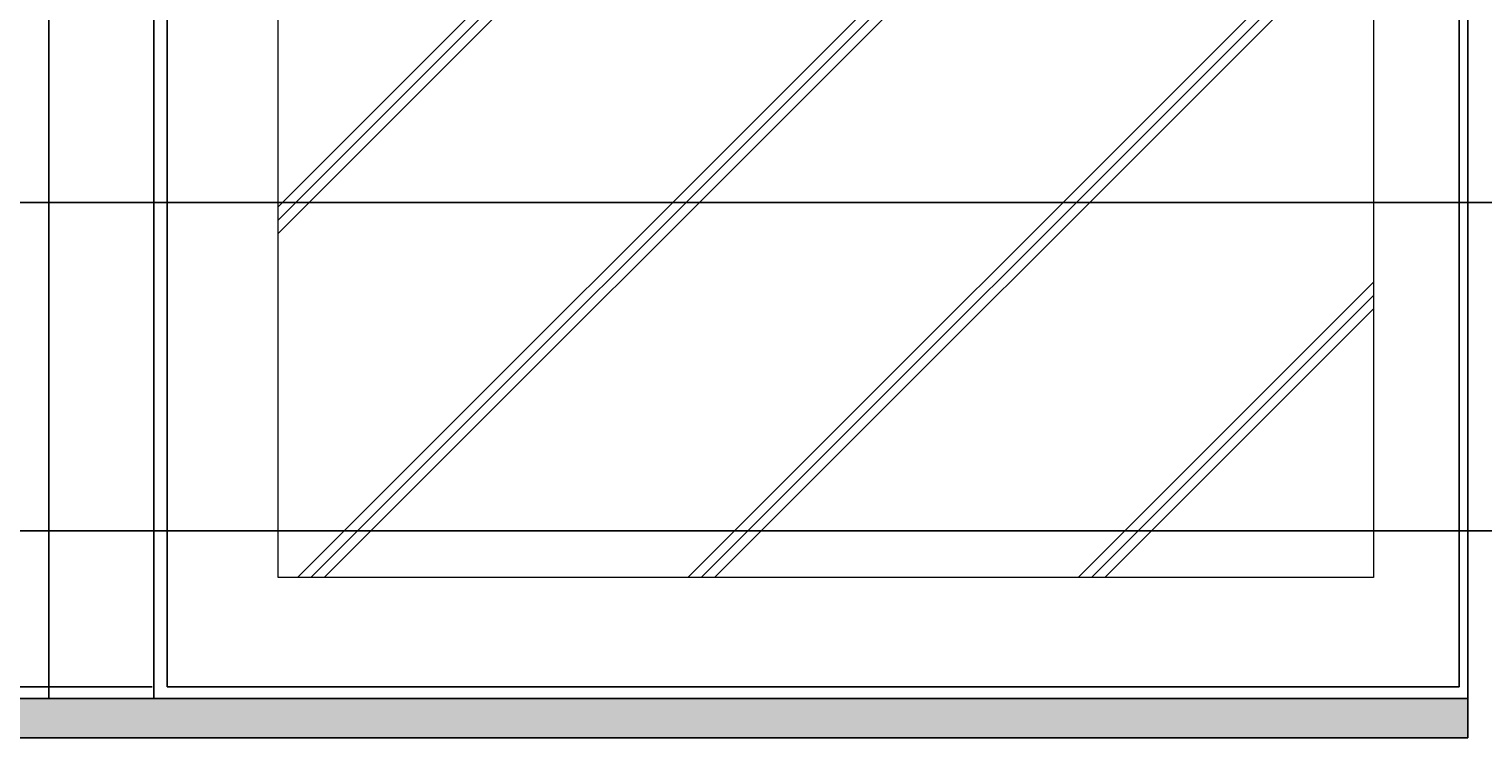
# Model space of a CAD drawing. Units: millimetres. Extents: x 2332 to 5836, y -853 to 2199.
# Tile 3 of 16: x 3088 to 3641, y 753 to 1023. Entities that reach past the tile are written whole.
import ezdxf

# ---------------------------------------------------------------- set-up
doc = ezdxf.new("R2010")
doc.units = ezdxf.units.MM
doc.layers.get('0').update_dxf_attribs({"color": 8})
for name, color, linetype, lineweight in [('A-ANNO-DIMS', 2, 'Continuous', 18), ('A-CSWK-GLAZ', 7, 'Continuous', 18), ('A-CSWK-PATT', 40, 'Continuous', 13), ('A-GLAZ-PATT', 4, 'Continuous', 13), ('SHELF', 40, 'Continuous', 25)]:
    doc.layers.add(name, color=color, linetype=linetype, lineweight=lineweight)
doc.styles.get("Standard").update_dxf_attribs({"font": 'arial.ttf'})
doc.dimstyles.new('ISO-25', dxfattribs={"dimtxt": 2.5, "dimasz": 2.5, "dimexe": 1.25, "dimexo": 0.625, "dimtad": 1, "dimtxsty": 'Standard', "dimcen": 2.5, "dimadec": 0, "dimazin": 0, "dimtfac": 1, "dimtmove": 0, "dimatfit": 3, "dimfxl": 1, "dimarcsym": 0})

# ---------------------------------------------------------------- blocks, each defined once
blk = doc.blocks.new('CAB-END-STILE')
blk.add_line((113.09, 1240), (113.09, 0))
blk = doc.blocks.new('CAB-GLAZED-FACE-FRAME')
for p, q in [((500, 575.53), (0, 575.53)), ((5, 575.53), (5, 0)), ((496.71, 0), (496.71, 575.53)), ((5, 0), (496.71, 0))]:
    blk.add_line(p, q)
blk = doc.blocks.new('*D13')
at = {"layer": 'A-ANNO-DIMS', "color": 0, "lineweight": -2, "transparency": 16777216}
for p, q in [((3134.41, 1347.8), (3047.46, 1347.8)), ((3048.71, 774.77), (3048.71, 1345.3)), ((3134.41, 772.27), (3047.46, 772.27))]:
    blk.add_line(p, q, dxfattribs=at)
at = {"layer": 'A-ANNO-DIMS', "color": 0, "transparency": 16777216}
for points in [[(3048.29, 1345.3), (3049.13, 1345.3), (3048.71, 1347.8)], [(3048.29, 774.77), (3049.13, 774.77), (3048.71, 772.27)]]:
    blk.add_solid(points, dxfattribs=at)
at = {"layer": 'Defpoints', "color": 0, "transparency": 16777216}
for p in [(3048.71, 1347.8), (3135.04, 1347.8), (3135.04, 772.27)]:
    blk.add_point(p, dxfattribs=at)
at = {"layer": 'A-ANNO-DIMS', "color": 0, "transparency": 16777216, "insert": (3046.79, 1060.04), "char_height": 2.5, "attachment_point": 5, "rotation": 90}
blk.add_mtext('GLAZED FRAME 576 TYP.', dxfattribs=at)
blk = doc.blocks.new('*D28')
at = {"layer": 'A-ANNO-DIMS', "color": 0, "lineweight": -2, "transparency": 16777216}
for p, q in [((3772.04, 956.62), (2334.14, 956.62)), ((2335.39, 834.12), (2335.39, 954.12)), ((3772.04, 831.62), (2334.14, 831.62))]:
    blk.add_line(p, q, dxfattribs=at)
at = {"layer": 'A-ANNO-DIMS', "color": 0, "transparency": 16777216}
for points in [[(2334.97, 954.12), (2335.81, 954.12), (2335.39, 956.62)], [(2334.97, 834.12), (2335.81, 834.12), (2335.39, 831.62)]]:
    blk.add_solid(points, dxfattribs=at)
at = {"layer": 'Defpoints', "color": 0, "transparency": 16777216}
for p in [(2335.39, 956.62), (3772.66, 956.62), (3772.66, 831.62)]:
    blk.add_point(p, dxfattribs=at)
at = {"layer": 'A-ANNO-DIMS', "color": 0, "transparency": 16777216, "insert": (2333.49, 894.12), "char_height": 2.5, "attachment_point": 5, "rotation": 90}
blk.add_mtext('125', dxfattribs=at)

msp = doc.modelspace()

# ---------------------------------------------------------------- hatches: boundary and pattern name
at = {"layer": 'A-CSWK-PATT'}
h = msp.add_hatch(color=256, dxfattribs=at)
h.dxf.hatch_style = 1
h.paths.add_polyline_path([(3635.04, 767.803), (3135.04, 767.803), (3095.04, 767.803), (2798.91, 767.803), (2798.91, 752.803), (3635.04, 752.803)])
at = {"layer": 'A-GLAZ-PATT'}
h = msp.add_hatch(dxfattribs=at)
h.set_pattern_fill('JIS_RC_15', color=256, scale=7)
h.paths.add_polyline_path([(3599.069, 1324.883), (3182.349, 1324.883), (3182.349, 1072.803), (3599.069, 1072.803)])
h.paths.add_polyline_path([(3599.069, 1042.803), (3182.349, 1042.803), (3182.349, 813.86), (3599.069, 813.86)])

# ---------------------------------------------------------------- linework, layer by layer
at = {"layer": 'A-CSWK-GLAZ'}
msp.add_lwpolyline([(3599.069, 1042.803), (3599.069, 813.86), (3182.349, 813.86), (3182.349, 1042.803)], dxfattribs=at)
at = {"layer": 'SHELF'}
for p, q in [((3135.04, 1967.803), (3135.04, 767.803)), ((3635.04, 767.803), (3635.04, 1967.803)), ((3095.04, 767.803), (2745.04, 767.803)), ((3135.04, 767.803), (3095.04, 767.803)), ((3135.04, 767.803), (3635.04, 767.803)), ((3635.04, 767.803), (3635.04, 752.803)), ((3635.04, 752.803), (2798.91, 752.803))]:
    msp.add_line(p, q, dxfattribs=at)

# ---------------------------------------------------------------- block references
for name, p in [('CAB-END-STILE', (2981.95, 767.803)), ('CAB-GLAZED-FACE-FRAME', (3135.04, 772.269))]:
    msp.add_blockref(name, p, dxfattribs=at)

# ---------------------------------------------------------------- dimensions: what is measured, and where the dimension line sits
at = {"layer": 'A-ANNO-DIMS'}
dim = msp.add_linear_dim(base=(3048.71, 1347.803), p1=(3135.04, 772.269), p2=(3135.04, 1347.803), angle=90, text='GLAZED FRAME <> TYP.', dimstyle='ISO-25', override={"dimdec": 0, "dimlfac": 1, "dimrnd": 0, "dimzin": 0, "dimdsep": 46, "dimlunit": 2}, dxfattribs=at)
dim.commit()
dim.dimension.update_dxf_attribs({"geometry": '*D13', "text_midpoint": (3046.792, 1060.036)})
dim = msp.add_linear_dim(base=(2335.39, 956.62), p1=(3772.661, 831.62), p2=(3772.661, 956.62), angle=90, dimstyle='ISO-25', override={"dimdec": 0, "dimlfac": 1, "dimrnd": 0, "dimzin": 0, "dimdsep": 46, "dimlunit": 2}, dxfattribs=at)
dim.commit()
dim.dimension.update_dxf_attribs({"geometry": '*D28', "text_midpoint": (2333.488, 894.12)})

doc.saveas('drawing.dxf')
